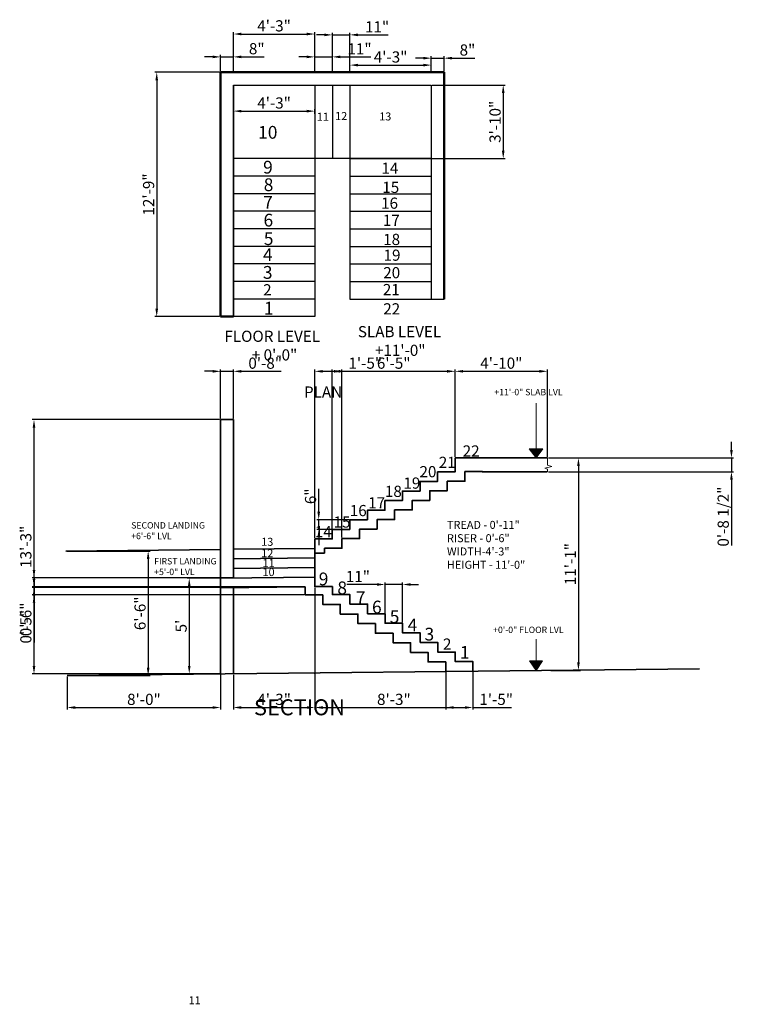
# Model space of a CAD drawing. Units: inches. Extents: x 2958 to 3410, y 1262 to 1879.
import ezdxf

# ---------------------------------------------------------------- set-up
doc = ezdxf.new("R2010")
doc.units = ezdxf.units.IN
for name, color, linetype, lineweight in [('A-ANNO-DIMS', 2, 'Continuous', 18), ('A-ANNO-SYMB', 2, 'Continuous', 18), ('A-ANNO-TEXT', 7, 'Continuous', 18), ('A-FLOR-STRS', 3, 'Continuous', 25), ('A-SECT', 7, 'Continuous', 35), ('A-WALL', 7, 'Continuous', 50)]:
    doc.layers.add(name, color=color, linetype=linetype, lineweight=lineweight)
doc.styles.get("Standard").update_dxf_attribs({"font": 'arial.ttf'})
doc.dimstyles.new('ISO-25', dxfattribs={"dimtxt": 7, "dimasz": 5, "dimexe": 1.25, "dimexo": 0.625, "dimtad": 1, "dimdec": 0, "dimlunit": 3, "dimtxsty": 'Standard', "dimcen": 2.5, "dimadec": 0, "dimazin": 0, "dimtfac": 1, "dimtdec": 0, "dimtmove": 0, "dimatfit": 3, "dimfxl": 1, "dimarcsym": 0})

# ---------------------------------------------------------------- blocks, each defined once
blk = doc.blocks.new('*D1')
at = {"layer": 'A-ANNO-DIMS', "color": 0, "lineweight": -2, "transparency": 16777216}
for p, q in [((3083.14, 1845.78), (3042.51, 1845.78)), ((3043.76, 1840.78), (3043.76, 1697.78)), ((3083.14, 1692.78), (3042.51, 1692.78))]:
    blk.add_line(p, q, dxfattribs=at)
at = {"layer": 'A-ANNO-DIMS', "color": 0, "transparency": 16777216}
for points in [[(3042.92, 1840.78), (3044.59, 1840.78), (3043.76, 1845.78)], [(3042.92, 1697.78), (3044.59, 1697.78), (3043.76, 1692.78)]]:
    blk.add_solid(points, dxfattribs=at)
at = {"layer": 'Defpoints', "color": 0, "transparency": 16777216}
for p in [(3083.76, 1845.78), (3043.76, 1692.78), (3083.76, 1692.78)]:
    blk.add_point(p, dxfattribs=at)
at = {"layer": 'A-ANNO-DIMS', "color": 0, "transparency": 16777216, "insert": (3039.56, 1769.28), "char_height": 7, "attachment_point": 5, "rotation": 90}
blk.add_mtext('12\'-9"', dxfattribs=at)
blk = doc.blocks.new('*D2')
at = {"layer": 'A-ANNO-DIMS', "color": 0, "lineweight": -2, "transparency": 16777216}
for p, q in [((3216.39, 1837.78), (3262.07, 1837.78)), ((3260.82, 1832.78), (3260.82, 1796.78)), ((3216.39, 1791.78), (3262.07, 1791.78))]:
    blk.add_line(p, q, dxfattribs=at)
at = {"layer": 'A-ANNO-DIMS', "color": 0, "transparency": 16777216}
for points in [[(3259.99, 1832.78), (3261.65, 1832.78), (3260.82, 1837.78)], [(3259.99, 1796.78), (3261.65, 1796.78), (3260.82, 1791.78)]]:
    blk.add_solid(points, dxfattribs=at)
at = {"layer": 'Defpoints', "color": 0, "transparency": 16777216}
for p in [(3215.76, 1837.78), (3215.76, 1791.78), (3260.82, 1791.78)]:
    blk.add_point(p, dxfattribs=at)
at = {"layer": 'A-ANNO-DIMS', "color": 0, "transparency": 16777216, "insert": (3256.62, 1814.78), "char_height": 7, "attachment_point": 5, "rotation": 90}
blk.add_mtext('3\'-10"', dxfattribs=at)
blk = doc.blocks.new('*D3')
at = {"layer": 'A-ANNO-DIMS', "color": 0, "lineweight": -2, "transparency": 16777216}
for p, q in [((3091.76, 1819.79), (3091.76, 1822.73)), ((3096.76, 1821.48), (3137.76, 1821.48)), ((3142.76, 1819.79), (3142.76, 1822.73))]:
    blk.add_line(p, q, dxfattribs=at)
at = {"layer": 'A-ANNO-DIMS', "color": 0, "transparency": 16777216}
for points in [[(3096.76, 1822.31), (3096.76, 1820.65), (3091.76, 1821.48)], [(3137.76, 1822.31), (3137.76, 1820.65), (3142.76, 1821.48)]]:
    blk.add_solid(points, dxfattribs=at)
at = {"layer": 'Defpoints', "color": 0, "transparency": 16777216}
for p in [(3091.76, 1819.16), (3142.76, 1821.48), (3142.76, 1819.16)]:
    blk.add_point(p, dxfattribs=at)
at = {"layer": 'A-ANNO-DIMS', "color": 0, "transparency": 16777216, "insert": (3117.26, 1825.68), "char_height": 7, "attachment_point": 5}
blk.add_mtext('4\'-3"', dxfattribs=at)
blk = doc.blocks.new('*D4')
at = {"layer": 'A-ANNO-DIMS', "color": 0, "lineweight": -2, "transparency": 16777216}
for p, q in [((3083.76, 1846.4), (3083.76, 1856.7)), ((3091.76, 1846.4), (3091.76, 1856.7)), ((3078.76, 1855.45), (3073.76, 1855.45)), ((3083.76, 1855.45), (3091.76, 1855.45)), ((3096.76, 1855.45), (3111.07, 1855.45))]:
    blk.add_line(p, q, dxfattribs=at)
at = {"layer": 'A-ANNO-DIMS', "color": 0, "transparency": 16777216}
for points in [[(3078.76, 1856.29), (3078.76, 1854.62), (3083.76, 1855.45)], [(3096.76, 1856.29), (3096.76, 1854.62), (3091.76, 1855.45)]]:
    blk.add_solid(points, dxfattribs=at)
at = {"layer": 'Defpoints', "color": 0, "transparency": 16777216}
for p in [(3091.76, 1855.45), (3083.76, 1845.78), (3091.76, 1845.78)]:
    blk.add_point(p, dxfattribs=at)
at = {"layer": 'A-ANNO-DIMS', "color": 0, "transparency": 16777216, "insert": (3106.41, 1859.65), "char_height": 7, "attachment_point": 5}
blk.add_mtext('8"', dxfattribs=at)
blk = doc.blocks.new('*D5')
at = {"layer": 'A-ANNO-DIMS', "color": 0, "lineweight": -2, "transparency": 16777216}
for p, q in [((3091.76, 1846.4), (3091.76, 1871.01)), ((3096.76, 1869.76), (3137.76, 1869.76)), ((3142.76, 1846.4), (3142.76, 1871.01))]:
    blk.add_line(p, q, dxfattribs=at)
at = {"layer": 'A-ANNO-DIMS', "color": 0, "transparency": 16777216}
for points in [[(3096.76, 1870.6), (3096.76, 1868.93), (3091.76, 1869.76)], [(3137.76, 1870.6), (3137.76, 1868.93), (3142.76, 1869.76)]]:
    blk.add_solid(points, dxfattribs=at)
at = {"layer": 'Defpoints', "color": 0, "transparency": 16777216}
for p in [(3142.76, 1869.76), (3091.76, 1845.78), (3142.76, 1845.78)]:
    blk.add_point(p, dxfattribs=at)
at = {"layer": 'A-ANNO-DIMS', "color": 0, "transparency": 16777216, "insert": (3117.26, 1873.97), "char_height": 7, "attachment_point": 5}
blk.add_mtext('4\'-3"', dxfattribs=at)
blk = doc.blocks.new('*D6')
at = {"layer": 'A-ANNO-DIMS', "color": 0, "lineweight": -2, "transparency": 16777216}
for p, q in [((3142.76, 1846.4), (3142.76, 1856.69)), ((3153.76, 1846.4), (3153.76, 1856.69)), ((3137.76, 1855.44), (3132.76, 1855.44)), ((3142.76, 1855.44), (3153.76, 1855.44)), ((3158.76, 1855.44), (3177.84, 1855.44))]:
    blk.add_line(p, q, dxfattribs=at)
at = {"layer": 'A-ANNO-DIMS', "color": 0, "transparency": 16777216}
for points in [[(3137.76, 1856.27), (3137.76, 1854.61), (3142.76, 1855.44)], [(3158.76, 1856.27), (3158.76, 1854.61), (3153.76, 1855.44)]]:
    blk.add_solid(points, dxfattribs=at)
at = {"layer": 'Defpoints', "color": 0, "transparency": 16777216}
for p in [(3153.76, 1855.44), (3142.76, 1845.78), (3153.76, 1845.78)]:
    blk.add_point(p, dxfattribs=at)
at = {"layer": 'A-ANNO-DIMS', "color": 0, "transparency": 16777216, "insert": (3170.8, 1859.58), "char_height": 7, "attachment_point": 5}
blk.add_mtext('11"', dxfattribs=at)
blk = doc.blocks.new('*D7')
at = {"layer": 'A-ANNO-DIMS', "color": 0, "lineweight": -2, "transparency": 16777216}
for p, q in [((3148.76, 1869.23), (3143.76, 1869.23)), ((3153.76, 1846.4), (3153.76, 1870.48)), ((3153.76, 1869.23), (3164.76, 1869.23)), ((3164.76, 1846.4), (3164.76, 1870.48)), ((3169.76, 1869.23), (3188.84, 1869.23))]:
    blk.add_line(p, q, dxfattribs=at)
at = {"layer": 'A-ANNO-DIMS', "color": 0, "transparency": 16777216}
for points in [[(3148.76, 1870.06), (3148.76, 1868.4), (3153.76, 1869.23)], [(3169.76, 1870.06), (3169.76, 1868.4), (3164.76, 1869.23)]]:
    blk.add_solid(points, dxfattribs=at)
at = {"layer": 'Defpoints', "color": 0, "transparency": 16777216}
for p in [(3164.76, 1869.23), (3153.76, 1845.78), (3164.76, 1845.78)]:
    blk.add_point(p, dxfattribs=at)
at = {"layer": 'A-ANNO-DIMS', "color": 0, "transparency": 16777216, "insert": (3181.8, 1873.37), "char_height": 7, "attachment_point": 5}
blk.add_mtext('11"', dxfattribs=at)
blk = doc.blocks.new('*D8')
at = {"layer": 'A-ANNO-DIMS', "color": 0, "lineweight": -2, "transparency": 16777216}
for p, q in [((3164.76, 1846.4), (3164.76, 1851.54)), ((3169.76, 1850.29), (3210.76, 1850.29)), ((3215.76, 1846.4), (3215.76, 1851.54))]:
    blk.add_line(p, q, dxfattribs=at)
at = {"layer": 'A-ANNO-DIMS', "color": 0, "transparency": 16777216}
for points in [[(3169.76, 1851.12), (3169.76, 1849.46), (3164.76, 1850.29)], [(3210.76, 1851.12), (3210.76, 1849.46), (3215.76, 1850.29)]]:
    blk.add_solid(points, dxfattribs=at)
at = {"layer": 'Defpoints', "color": 0, "transparency": 16777216}
for p in [(3215.76, 1850.29), (3164.76, 1845.78), (3215.76, 1845.78)]:
    blk.add_point(p, dxfattribs=at)
at = {"layer": 'A-ANNO-DIMS', "color": 0, "transparency": 16777216, "insert": (3190.26, 1854.49), "char_height": 7, "attachment_point": 5}
blk.add_mtext('4\'-3"', dxfattribs=at)
blk = doc.blocks.new('*D9')
at = {"layer": 'A-ANNO-DIMS', "color": 0, "lineweight": -2, "transparency": 16777216}
for p, q in [((3215.76, 1846.4), (3215.76, 1855.9)), ((3223.76, 1846.4), (3223.76, 1855.9)), ((3210.76, 1854.65), (3205.76, 1854.65)), ((3215.76, 1854.65), (3223.76, 1854.65)), ((3228.76, 1854.65), (3243.07, 1854.65))]:
    blk.add_line(p, q, dxfattribs=at)
at = {"layer": 'A-ANNO-DIMS', "color": 0, "transparency": 16777216}
for points in [[(3210.76, 1855.48), (3210.76, 1853.81), (3215.76, 1854.65)], [(3228.76, 1855.48), (3228.76, 1853.81), (3223.76, 1854.65)]]:
    blk.add_solid(points, dxfattribs=at)
at = {"layer": 'Defpoints', "color": 0, "transparency": 16777216}
for p in [(3223.76, 1854.65), (3215.76, 1845.78), (3223.76, 1845.78)]:
    blk.add_point(p, dxfattribs=at)
at = {"layer": 'A-ANNO-DIMS', "color": 0, "transparency": 16777216, "insert": (3238.41, 1858.85), "char_height": 7, "attachment_point": 5}
blk.add_mtext('8"', dxfattribs=at)
blk = doc.blocks.new('*D11')
at = {"layer": 'A-ANNO-DIMS', "color": 0, "lineweight": -2, "transparency": 16777216}
for p, q in [((3145.23, 1570.61), (3145.23, 1584.94)), ((3164.07, 1565.61), (3143.98, 1565.61)), ((3145.23, 1559.61), (3145.23, 1565.61)), ((3164.07, 1559.61), (3143.98, 1559.61)), ((3145.23, 1554.61), (3145.23, 1549.61))]:
    blk.add_line(p, q, dxfattribs=at)
at = {"layer": 'A-ANNO-DIMS', "color": 0, "transparency": 16777216}
for points in [[(3144.4, 1570.61), (3146.07, 1570.61), (3145.23, 1565.61)], [(3144.4, 1554.61), (3146.07, 1554.61), (3145.23, 1559.61)]]:
    blk.add_solid(points, dxfattribs=at)
at = {"layer": 'Defpoints', "color": 0, "transparency": 16777216}
for p in [(3145.23, 1565.61), (3164.7, 1565.61), (3164.7, 1559.61)]:
    blk.add_point(p, dxfattribs=at)
at = {"layer": 'A-ANNO-DIMS', "color": 0, "transparency": 16777216, "insert": (3141.03, 1580.28), "char_height": 7, "attachment_point": 5, "rotation": 90}
blk.add_mtext('6"', dxfattribs=at)
blk = doc.blocks.new('*D12')
at = {"layer": 'A-ANNO-DIMS', "color": 0, "lineweight": -2, "transparency": 16777216}
for p, q in [((3181.81, 1525.07), (3162.74, 1525.07)), ((3186.81, 1501.4), (3186.81, 1526.32)), ((3197.81, 1525.07), (3186.81, 1525.07)), ((3197.81, 1501.4), (3197.81, 1526.32)), ((3202.81, 1525.07), (3207.81, 1525.07))]:
    blk.add_line(p, q, dxfattribs=at)
at = {"layer": 'A-ANNO-DIMS', "color": 0, "transparency": 16777216}
for points in [[(3181.81, 1525.9), (3181.81, 1524.24), (3186.81, 1525.07)], [(3202.81, 1525.9), (3202.81, 1524.24), (3197.81, 1525.07)]]:
    blk.add_solid(points, dxfattribs=at)
at = {"layer": 'Defpoints', "color": 0, "transparency": 16777216}
for p in [(3186.81, 1525.07), (3186.81, 1500.78), (3197.81, 1500.78)]:
    blk.add_point(p, dxfattribs=at)
at = {"layer": 'A-ANNO-DIMS', "color": 0, "transparency": 16777216, "insert": (3169.78, 1529.21), "char_height": 7, "attachment_point": 5}
blk.add_mtext('11"', dxfattribs=at)
blk = doc.blocks.new('*D13')
at = {"layer": 'A-ANNO-DIMS', "color": 0, "lineweight": -2, "transparency": 16777216}
for p, q in [((3083.14, 1529.06), (3062.87, 1529.06)), ((3064.12, 1524.06), (3064.12, 1474.06)), ((3083.14, 1469.06), (3062.87, 1469.06))]:
    blk.add_line(p, q, dxfattribs=at)
at = {"layer": 'A-ANNO-DIMS', "color": 0, "transparency": 16777216}
for points in [[(3063.29, 1524.06), (3064.95, 1524.06), (3064.12, 1529.06)], [(3063.29, 1474.06), (3064.95, 1474.06), (3064.12, 1469.06)]]:
    blk.add_solid(points, dxfattribs=at)
at = {"layer": 'Defpoints', "color": 0, "transparency": 16777216}
for p in [(3083.76, 1529.06), (3064.12, 1469.06), (3083.76, 1469.06)]:
    blk.add_point(p, dxfattribs=at)
at = {"layer": 'A-ANNO-DIMS', "color": 0, "transparency": 16777216, "insert": (3059.94, 1499.06), "char_height": 7, "attachment_point": 5, "rotation": 90}
blk.add_mtext("5'", dxfattribs=at)
blk = doc.blocks.new('*D14')
at = {"layer": 'A-ANNO-DIMS', "color": 0, "lineweight": -2, "transparency": 16777216}
for p, q in [((3289.17, 1604.32), (3309.2, 1604.32)), ((3307.95, 1599.32), (3307.95, 1476.3)), ((3290.61, 1471.3), (3309.2, 1471.3))]:
    blk.add_line(p, q, dxfattribs=at)
at = {"layer": 'A-ANNO-DIMS', "color": 0, "transparency": 16777216}
for points in [[(3307.12, 1599.32), (3308.78, 1599.32), (3307.95, 1604.32)], [(3307.12, 1476.3), (3308.78, 1476.3), (3307.95, 1471.3)]]:
    blk.add_solid(points, dxfattribs=at)
at = {"layer": 'Defpoints', "color": 0, "transparency": 16777216}
for p in [(3288.54, 1604.32), (3289.99, 1471.3), (3307.95, 1471.3)]:
    blk.add_point(p, dxfattribs=at)
at = {"layer": 'A-ANNO-DIMS', "color": 0, "transparency": 16777216, "insert": (3303.81, 1537.81), "char_height": 7, "attachment_point": 5, "rotation": 90}
blk.add_mtext('11\'-1"', dxfattribs=at)
blk = doc.blocks.new('*D15')
at = {"layer": 'A-ANNO-DIMS', "color": 0, "lineweight": -2, "transparency": 16777216}
for p, q in [((2987.46, 1546.01), (3039.64, 1546.01)), ((3038.39, 1541.01), (3038.39, 1473.01)), ((2988.31, 1468.01), (3039.64, 1468.01))]:
    blk.add_line(p, q, dxfattribs=at)
at = {"layer": 'A-ANNO-DIMS', "color": 0, "transparency": 16777216}
for points in [[(3037.55, 1541.01), (3039.22, 1541.01), (3038.39, 1546.01)], [(3037.55, 1473.01), (3039.22, 1473.01), (3038.39, 1468.01)]]:
    blk.add_solid(points, dxfattribs=at)
at = {"layer": 'Defpoints', "color": 0, "transparency": 16777216}
for p in [(2986.84, 1546.01), (2987.68, 1468.01), (3038.39, 1468.01)]:
    blk.add_point(p, dxfattribs=at)
at = {"layer": 'A-ANNO-DIMS', "color": 0, "transparency": 16777216, "insert": (3034.19, 1507.01), "char_height": 7, "attachment_point": 5, "rotation": 90}
blk.add_mtext('6\'-6"', dxfattribs=at)
blk = doc.blocks.new('*D18')
at = {"layer": 'A-ANNO-DIMS', "color": 0, "lineweight": -2, "transparency": 16777216}
for p, q in [((3078.76, 1658.55), (3073.76, 1658.55)), ((3083.76, 1628.91), (3083.76, 1659.8)), ((3083.76, 1658.55), (3091.76, 1658.55)), ((3091.76, 1628.91), (3091.76, 1659.8)), ((3096.76, 1658.55), (3121.62, 1658.55))]:
    blk.add_line(p, q, dxfattribs=at)
at = {"layer": 'A-ANNO-DIMS', "color": 0, "transparency": 16777216}
for points in [[(3078.76, 1659.39), (3078.76, 1657.72), (3083.76, 1658.55)], [(3096.76, 1659.39), (3096.76, 1657.72), (3091.76, 1658.55)]]:
    blk.add_solid(points, dxfattribs=at)
at = {"layer": 'Defpoints', "color": 0, "transparency": 16777216}
for p in [(3091.76, 1658.55), (3083.76, 1628.29), (3091.76, 1628.29)]:
    blk.add_point(p, dxfattribs=at)
at = {"layer": 'A-ANNO-DIMS', "color": 0, "transparency": 16777216, "insert": (3111.69, 1662.75), "char_height": 7, "attachment_point": 5}
blk.add_mtext('0\'-8"', dxfattribs=at)
blk = doc.blocks.new('*D19')
at = {"layer": 'A-ANNO-DIMS', "color": 0, "lineweight": -2, "transparency": 16777216}
for p, q in [((3083.14, 1628.29), (2965.61, 1628.29)), ((2966.86, 1474.06), (2966.86, 1623.29)), ((3083.14, 1469.06), (2965.61, 1469.06))]:
    blk.add_line(p, q, dxfattribs=at)
at = {"layer": 'A-ANNO-DIMS', "color": 0, "transparency": 16777216}
for points in [[(2966.03, 1623.29), (2967.69, 1623.29), (2966.86, 1628.29)], [(2966.03, 1474.06), (2967.69, 1474.06), (2966.86, 1469.06)]]:
    blk.add_solid(points, dxfattribs=at)
at = {"layer": 'Defpoints', "color": 0, "transparency": 16777216}
for p in [(2966.86, 1628.29), (3083.76, 1628.29), (3083.76, 1469.06)]:
    blk.add_point(p, dxfattribs=at)
at = {"layer": 'A-ANNO-DIMS', "color": 0, "transparency": 16777216, "insert": (2962.66, 1548.67), "char_height": 7, "attachment_point": 5, "rotation": 90}
blk.add_mtext('13\'-3"', dxfattribs=at)
blk = doc.blocks.new('*D20')
at = {"layer": 'A-ANNO-DIMS', "color": 0, "lineweight": -2, "transparency": 16777216}
for p, q in [((2987.68, 1467.39), (2987.68, 1446.79)), ((3083.76, 1468.43), (3083.76, 1446.79)), ((2992.68, 1448.04), (3078.76, 1448.04))]:
    blk.add_line(p, q, dxfattribs=at)
at = {"layer": 'A-ANNO-DIMS', "color": 0, "transparency": 16777216}
for points in [[(2992.68, 1448.87), (2992.68, 1447.21), (2987.68, 1448.04)], [(3078.76, 1448.87), (3078.76, 1447.21), (3083.76, 1448.04)]]:
    blk.add_solid(points, dxfattribs=at)
at = {"layer": 'Defpoints', "color": 0, "transparency": 16777216}
for p in [(2987.68, 1468.01), (3083.76, 1469.06), (3083.76, 1448.04)]:
    blk.add_point(p, dxfattribs=at)
at = {"layer": 'A-ANNO-DIMS', "color": 0, "transparency": 16777216, "insert": (3035.72, 1452.24), "char_height": 7, "attachment_point": 5}
blk.add_mtext('8\'-0"', dxfattribs=at)
blk = doc.blocks.new('*D21')
at = {"layer": 'A-ANNO-DIMS', "color": 0, "lineweight": -2, "transparency": 16777216}
for p, q in [((3142.83, 1523.08), (3142.83, 1446.79)), ((3091.76, 1468.43), (3091.76, 1446.79)), ((3096.76, 1448.04), (3137.83, 1448.04))]:
    blk.add_line(p, q, dxfattribs=at)
at = {"layer": 'A-ANNO-DIMS', "color": 0, "transparency": 16777216}
for points in [[(3096.76, 1448.87), (3096.76, 1447.21), (3091.76, 1448.04)], [(3137.83, 1448.87), (3137.83, 1447.21), (3142.83, 1448.04)]]:
    blk.add_solid(points, dxfattribs=at)
at = {"layer": 'Defpoints', "color": 0, "transparency": 16777216}
for p in [(3142.83, 1523.71), (3091.76, 1469.06), (3142.83, 1448.04)]:
    blk.add_point(p, dxfattribs=at)
at = {"layer": 'A-ANNO-DIMS', "color": 0, "transparency": 16777216, "insert": (3117.29, 1452.24), "char_height": 7, "attachment_point": 5}
blk.add_mtext('4\'-3"', dxfattribs=at)
blk = doc.blocks.new('*D22')
at = {"layer": 'A-ANNO-DIMS', "color": 0, "lineweight": -2, "transparency": 16777216}
for p, q in [((3142.83, 1523.08), (3142.83, 1446.79)), ((3241.81, 1470.15), (3241.81, 1446.79)), ((3147.83, 1448.04), (3236.81, 1448.04))]:
    blk.add_line(p, q, dxfattribs=at)
at = {"layer": 'A-ANNO-DIMS', "color": 0, "transparency": 16777216}
for points in [[(3147.83, 1448.87), (3147.83, 1447.21), (3142.83, 1448.04)], [(3236.81, 1448.87), (3236.81, 1447.21), (3241.81, 1448.04)]]:
    blk.add_solid(points, dxfattribs=at)
at = {"layer": 'Defpoints', "color": 0, "transparency": 16777216}
for p in [(3142.83, 1523.71), (3241.81, 1470.78), (3241.81, 1448.04)]:
    blk.add_point(p, dxfattribs=at)
at = {"layer": 'A-ANNO-DIMS', "color": 0, "transparency": 16777216, "insert": (3192.32, 1452.24), "char_height": 7, "attachment_point": 5}
blk.add_mtext('8\'-3"', dxfattribs=at)
blk = doc.blocks.new('*D23')
at = {"layer": 'A-ANNO-DIMS', "color": 0, "lineweight": -2, "transparency": 16777216}
for p, q in [((3224.77, 1469.97), (3224.77, 1446.79)), ((3241.81, 1470.15), (3241.81, 1446.79)), ((3229.77, 1448.04), (3236.81, 1448.04)), ((3241.81, 1448.04), (3266.01, 1448.04))]:
    blk.add_line(p, q, dxfattribs=at)
at = {"layer": 'A-ANNO-DIMS', "color": 0, "transparency": 16777216}
for points in [[(3229.77, 1448.87), (3229.77, 1447.21), (3224.77, 1448.04)], [(3236.81, 1448.87), (3236.81, 1447.21), (3241.81, 1448.04)]]:
    blk.add_solid(points, dxfattribs=at)
at = {"layer": 'Defpoints', "color": 0, "transparency": 16777216}
for p in [(3224.77, 1470.59), (3241.81, 1470.78), (3241.81, 1448.04)]:
    blk.add_point(p, dxfattribs=at)
at = {"layer": 'A-ANNO-DIMS', "color": 0, "transparency": 16777216, "insert": (3256.41, 1452.24), "char_height": 7, "attachment_point": 5}
blk.add_mtext('1\'-5"', dxfattribs=at)
blk = doc.blocks.new('*D24')
at = {"layer": 'A-ANNO-DIMS', "color": 0, "lineweight": -2, "transparency": 16777216}
for p, q in [((2966.86, 1534.15), (2966.86, 1539.15)), ((3091.14, 1529.15), (2965.61, 1529.15)), ((2966.86, 1529.15), (2966.86, 1523.15)), ((3091.14, 1523.15), (2965.61, 1523.15)), ((2966.86, 1518.15), (2966.86, 1493.29))]:
    blk.add_line(p, q, dxfattribs=at)
at = {"layer": 'A-ANNO-DIMS', "color": 0, "transparency": 16777216}
for points in [[(2966.03, 1534.15), (2967.69, 1534.15), (2966.86, 1529.15)], [(2966.03, 1518.15), (2967.69, 1518.15), (2966.86, 1523.15)]]:
    blk.add_solid(points, dxfattribs=at)
at = {"layer": 'Defpoints', "color": 0, "transparency": 16777216}
for p in [(3091.76, 1529.15), (2966.86, 1523.15), (3091.76, 1523.15)]:
    blk.add_point(p, dxfattribs=at)
at = {"layer": 'A-ANNO-DIMS', "color": 0, "transparency": 16777216, "insert": (2962.66, 1503.22), "char_height": 7, "attachment_point": 5, "rotation": 90}
blk.add_mtext('0\'-6"', dxfattribs=at)
blk = doc.blocks.new('*D25')
at = {"layer": 'A-ANNO-DIMS', "color": 0, "lineweight": -2, "transparency": 16777216}
for p, q in [((2966.86, 1528.58), (2966.86, 1533.58)), ((3136.15, 1523.58), (2965.61, 1523.58)), ((2966.86, 1523.58), (2966.86, 1518.59)), ((3136.14, 1518.59), (2965.61, 1518.59)), ((2966.86, 1513.59), (2966.86, 1488.74))]:
    blk.add_line(p, q, dxfattribs=at)
at = {"layer": 'A-ANNO-DIMS', "color": 0, "transparency": 16777216}
for points in [[(2966.03, 1528.58), (2967.69, 1528.58), (2966.86, 1523.58)], [(2966.03, 1513.59), (2967.69, 1513.59), (2966.86, 1518.59)]]:
    blk.add_solid(points, dxfattribs=at)
at = {"layer": 'Defpoints', "color": 0, "transparency": 16777216}
for p in [(3136.78, 1523.58), (2966.86, 1518.59), (3136.77, 1518.59)]:
    blk.add_point(p, dxfattribs=at)
at = {"layer": 'A-ANNO-DIMS', "color": 0, "transparency": 16777216, "insert": (2962.66, 1498.66), "char_height": 7, "attachment_point": 5, "rotation": 90}
blk.add_mtext('0\'-5"', dxfattribs=at)
blk = doc.blocks.new('*D26')
at = {"layer": 'A-ANNO-DIMS', "color": 0, "lineweight": -2, "transparency": 16777216}
for p, q in [((3153.7, 1560.23), (3153.7, 1659.8)), ((3158.7, 1658.55), (3225.7, 1658.55)), ((3230.7, 1604.95), (3230.7, 1659.8))]:
    blk.add_line(p, q, dxfattribs=at)
at = {"layer": 'A-ANNO-DIMS', "color": 0, "transparency": 16777216}
for points in [[(3158.7, 1659.39), (3158.7, 1657.72), (3153.7, 1658.55)], [(3225.7, 1659.39), (3225.7, 1657.72), (3230.7, 1658.55)]]:
    blk.add_solid(points, dxfattribs=at)
at = {"layer": 'Defpoints', "color": 0, "transparency": 16777216}
for p in [(3230.7, 1658.55), (3230.7, 1604.32), (3153.7, 1559.61)]:
    blk.add_point(p, dxfattribs=at)
at = {"layer": 'A-ANNO-DIMS', "color": 0, "transparency": 16777216, "insert": (3192.2, 1662.75), "char_height": 7, "attachment_point": 5}
blk.add_mtext('6\'-5"', dxfattribs=at)
blk = doc.blocks.new('*D27')
at = {"layer": 'A-ANNO-DIMS', "color": 0, "lineweight": -2, "transparency": 16777216}
for p, q in [((3230.7, 1604.95), (3230.7, 1659.8)), ((3235.7, 1658.55), (3283.54, 1658.55)), ((3288.54, 1604.95), (3288.54, 1659.8))]:
    blk.add_line(p, q, dxfattribs=at)
at = {"layer": 'A-ANNO-DIMS', "color": 0, "transparency": 16777216}
for points in [[(3235.7, 1659.39), (3235.7, 1657.72), (3230.7, 1658.55)], [(3283.54, 1659.39), (3283.54, 1657.72), (3288.54, 1658.55)]]:
    blk.add_solid(points, dxfattribs=at)
at = {"layer": 'Defpoints', "color": 0, "transparency": 16777216}
for p in [(3288.54, 1658.55), (3230.7, 1604.32), (3288.54, 1604.32)]:
    blk.add_point(p, dxfattribs=at)
at = {"layer": 'A-ANNO-DIMS', "color": 0, "transparency": 16777216, "insert": (3259.62, 1662.75), "char_height": 7, "attachment_point": 5}
blk.add_mtext('4\'-10"', dxfattribs=at)
blk = doc.blocks.new('*D28')
at = {"layer": 'A-ANNO-DIMS', "color": 0, "lineweight": -2, "transparency": 16777216}
for p, q in [((3142.76, 1554.23), (3142.76, 1659.8)), ((3147.76, 1658.55), (3154.79, 1658.55)), ((3159.79, 1554.4), (3159.79, 1659.8)), ((3159.79, 1658.55), (3183.99, 1658.55))]:
    blk.add_line(p, q, dxfattribs=at)
at = {"layer": 'A-ANNO-DIMS', "color": 0, "transparency": 16777216}
for points in [[(3147.76, 1659.39), (3147.76, 1657.72), (3142.76, 1658.55)], [(3154.79, 1659.39), (3154.79, 1657.72), (3159.79, 1658.55)]]:
    blk.add_solid(points, dxfattribs=at)
at = {"layer": 'Defpoints', "color": 0, "transparency": 16777216}
for p in [(3159.79, 1658.55), (3159.79, 1553.77), (3142.76, 1553.61)]:
    blk.add_point(p, dxfattribs=at)
at = {"layer": 'A-ANNO-DIMS', "color": 0, "transparency": 16777216, "insert": (3174.39, 1662.75), "char_height": 7, "attachment_point": 5}
blk.add_mtext('1\'-5"', dxfattribs=at)
blk = doc.blocks.new('*D29')
at = {"layer": 'A-ANNO-DIMS', "color": 0, "lineweight": -2, "transparency": 16777216}
for p, q in [((3403.79, 1609.32), (3403.79, 1614.32)), ((3289.17, 1604.32), (3405.04, 1604.32)), ((3403.79, 1604.32), (3403.79, 1595.67)), ((3289.26, 1595.67), (3405.04, 1595.67)), ((3403.79, 1590.67), (3403.79, 1549.5))]:
    blk.add_line(p, q, dxfattribs=at)
at = {"layer": 'A-ANNO-DIMS', "color": 0, "transparency": 16777216}
for points in [[(3402.95, 1609.32), (3404.62, 1609.32), (3403.79, 1604.32)], [(3402.95, 1590.67), (3404.62, 1590.67), (3403.79, 1595.67)]]:
    blk.add_solid(points, dxfattribs=at)
at = {"layer": 'Defpoints', "color": 0, "transparency": 16777216}
for p in [(3288.54, 1604.32), (3288.63, 1595.67), (3403.79, 1595.67)]:
    blk.add_point(p, dxfattribs=at)
at = {"layer": 'A-ANNO-DIMS', "color": 0, "transparency": 16777216, "insert": (3399.54, 1567.59), "char_height": 7, "attachment_point": 5, "rotation": 90}
blk.add_mtext('0\'-8 1/2"', dxfattribs=at)

msp = doc.modelspace()

# ---------------------------------------------------------------- hatches: boundary and pattern name
at = {"layer": 'A-ANNO-SYMB'}
h = msp.add_hatch(color=256, dxfattribs=at)
h.dxf.hatch_style = 1
h.paths.add_polyline_path([(3281.39, 1604.32), (3281.39, 1610.09), (3277.15, 1610.09)])
h = msp.add_hatch(color=256, dxfattribs=at)
h.dxf.hatch_style = 1
h.paths.add_polyline_path([(3281.39, 1610.09), (3281.39, 1604.32), (3285.63, 1610.09)])
h = msp.add_hatch(color=256, dxfattribs=at)
h.dxf.hatch_style = 1
h.paths.add_polyline_path([(3281.39, 1477.29), (3277.33, 1477.29), (3281.39, 1471.23)])
h = msp.add_hatch(color=256, dxfattribs=at)
h.dxf.hatch_style = 1
h.paths.add_polyline_path([(3284.97, 1476.51), (3285.49, 1477.29), (3281.39, 1477.29), (3281.39, 1471.23), (3281.4, 1471.22)])

# ---------------------------------------------------------------- linework, layer by layer
for p, q in [((3281.39, 1604.32), (3281.39, 1638.58)), ((3281.39, 1604.32), (3277.15, 1610.09)), ((3277.15, 1610.09), (3285.63, 1610.09)), ((3281.39, 1604.32), (3285.63, 1610.09)), ((3281.39, 1604.32), (3281.39, 1604.32)), ((3288.54, 1604.32), (3288.54, 1599.77)), ((3291.35, 1598.97), (3286.82, 1598.01)), ((3286.82, 1598.01), (3288.63, 1597.26)), ((3288.54, 1599.77), (3291.35, 1598.97)), ((3288.63, 1597.26), (3288.63, 1595.67)), ((3281.39, 1471.21), (3281.39, 1490.93)), ((3281.41, 1471.19), (3277.33, 1477.29)), ((3277.33, 1477.29), (3285.49, 1477.29)), ((3281.39, 1471.21), (3285.49, 1477.28)), ((3281.41, 1471.19), (3285.49, 1477.29))]:
    msp.add_line(p, q, dxfattribs=at)
at = {"layer": 'A-FLOR-STRS'}
for p, q in [((3091.76, 1692.78), (3091.76, 1837.78)), ((3091.76, 1837.78), (3142.76, 1837.78)), ((3091.76, 1837.78), (3091.76, 1692.78)), ((3142.76, 1837.78), (3142.76, 1692.78)), ((3142.76, 1837.78), (3153.76, 1837.78)), ((3142.76, 1837.78), (3142.76, 1692.78)), ((3153.76, 1837.78), (3164.76, 1837.78)), ((3153.76, 1837.78), (3153.76, 1791.78)), ((3164.76, 1837.78), (3215.76, 1837.78)), ((3164.76, 1837.78), (3164.76, 1703.78)), ((3215.76, 1837.78), (3215.76, 1703.78)), ((3215.76, 1791.78), (3091.76, 1791.78)), ((3164.76, 1791.78), (3215.76, 1791.78)), ((3142.76, 1780.78), (3091.76, 1780.78)), ((3164.76, 1780.78), (3215.76, 1780.78)), ((3142.76, 1769.78), (3091.76, 1769.78)), ((3164.76, 1769.78), (3215.76, 1769.78)), ((3142.76, 1758.78), (3091.76, 1758.78)), ((3164.76, 1758.78), (3215.76, 1758.78)), ((3142.76, 1747.78), (3091.76, 1747.78)), ((3164.76, 1747.78), (3215.76, 1747.78)), ((3142.76, 1736.78), (3091.76, 1736.78)), ((3164.76, 1736.78), (3215.76, 1736.78)), ((3142.76, 1725.78), (3091.76, 1725.78)), ((3164.76, 1725.78), (3215.76, 1725.78)), ((3142.76, 1714.78), (3091.76, 1714.78)), ((3164.76, 1714.78), (3215.76, 1714.78)), ((3142.76, 1703.78), (3091.76, 1703.78)), ((3164.76, 1703.78), (3223.76, 1703.78)), ((3142.76, 1692.78), (3091.76, 1692.78))]:
    msp.add_line(p, q, dxfattribs=at)
at = {"layer": 'A-SECT'}
for p, q in [((3083.76, 1628.29), (3083.76, 1469.06)), ((3083.76, 1628.29), (3091.76, 1628.29)), ((3091.76, 1628.29), (3091.76, 1529.15)), ((3230.7, 1604.32), (3288.54, 1604.32)), ((3230.7, 1601.61), (3230.7, 1604.32)), ((3247.7, 1595.67), (3288.41, 1595.67)), ((3083.4, 1562.06), (3083.76, 1562.07)), ((3083.52, 1551.06), (3083.76, 1551.06)), ((3091.76, 1547.15), (3142.76, 1547.71)), ((3142.7, 1551.71), (3142.76, 1551.71)), ((3142.76, 1553.61), (3142.76, 1529.71)), ((3148.79, 1544.77), (3148.79, 1547.77)), ((2986.84, 1546.01), (3083.76, 1547.06)), ((3091.76, 1541.15), (3142.63, 1541.7)), ((3142.76, 1544.71), (3148.79, 1544.77)), ((3142.76, 1544.71), (3142.79, 1544.71)), ((3083.63, 1541.06), (3083.76, 1541.06)), ((3083.64, 1540.06), (3083.76, 1540.06)), ((3091.76, 1535.15), (3142.7, 1535.7)), ((3083.7, 1535.06), (3083.76, 1535.06)), ((3083.76, 1529.06), (3142.76, 1529.71)), ((3142.76, 1529.71), (3142.83, 1523.71)), ((3083.76, 1523.06), (3136.77, 1523.64)), ((3091.76, 1523.15), (3091.76, 1469.06)), ((3136.78, 1523.58), (3125.78, 1523.58)), ((3142.83, 1523.71), (3153.81, 1523.83)), ((3153.83, 1523.77), (3142.83, 1523.77)), ((2987.68, 1468.01), (3383.81, 1472.32)), ((3142.76, 1469.7), (3142.76, 1469.06))]:
    msp.add_line(p, q, dxfattribs=at)
for points in [[(3142.7, 1547.61), (3142.7, 1553.61), (3153.7, 1553.61), (3153.7, 1559.61), (3164.7, 1559.61), (3164.7, 1565.61), (3175.7, 1565.61), (3175.7, 1571.61), (3186.7, 1571.61), (3186.7, 1577.61), (3197.7, 1577.61), (3197.7, 1583.61), (3208.7, 1583.61), (3208.7, 1589.61), (3219.7, 1589.61), (3219.7, 1595.61), (3230.7, 1595.61), (3230.7, 1601.61)], [(3148.79, 1547.77), (3159.79, 1547.77), (3159.79, 1553.77), (3170.79, 1553.77), (3170.79, 1559.77), (3181.79, 1559.77), (3181.79, 1565.77), (3192.79, 1565.77), (3192.79, 1571.77), (3203.79, 1571.77), (3203.79, 1577.77), (3214.79, 1577.77), (3214.79, 1583.77), (3225.79, 1583.77), (3225.79, 1589.77), (3236.79, 1589.77), (3236.79, 1595.77), (3247.79, 1595.77)], [(3224.77, 1470.59), (3224.77, 1476.59), (3213.77, 1476.59), (3213.77, 1482.59), (3202.77, 1482.59), (3202.77, 1488.59), (3191.77, 1488.59), (3191.77, 1494.59), (3180.77, 1494.59), (3180.77, 1500.59), (3169.77, 1500.59), (3169.77, 1506.59), (3158.77, 1506.59), (3158.77, 1512.59), (3147.77, 1512.59), (3147.77, 1518.59), (3136.77, 1518.59), (3136.77, 1523.64)], [(3241.81, 1470.78), (3241.81, 1476.78), (3230.81, 1476.78), (3230.81, 1482.78), (3219.81, 1482.78), (3219.81, 1488.78), (3208.81, 1488.78), (3208.81, 1494.78), (3197.81, 1494.78), (3197.81, 1500.78), (3186.81, 1500.78), (3186.81, 1506.78), (3175.81, 1506.78), (3175.81, 1512.78), (3164.81, 1512.78), (3164.81, 1518.78), (3153.81, 1518.78), (3153.81, 1523.83)]]:
    msp.add_lwpolyline(points, dxfattribs=at)
at = {"layer": 'A-WALL'}
for p, q in [((3083.76, 1845.78), (3083.76, 1692.78)), ((3223.76, 1845.78), (3083.76, 1845.78)), ((3223.76, 1703.78), (3223.76, 1845.78)), ((3083.76, 1692.78), (3091.76, 1692.78))]:
    msp.add_line(p, q, dxfattribs=at)

# ---------------------------------------------------------------- texts
at = {"layer": 'A-ANNO-TEXT', "attachment_point": 1}
for s, width, heights, insert, char_height in [('11', 41.8662, [0], (3144.03, 1820.48), 5), ('12', 41.8662, [0], (3155.51, 1820.92), 5), ('13', 41.8662, [0], (3183.12, 1820.65), 5), ('10', 41.8662, [0], (3107.25, 1812.21), 8), ('9', 41.8662, [0], (3110.4, 1790.37), 8), ('14', 41.8662, [0], (3184.52, 1789.25), 7), ('8', 41.8662, [0], (3110.76, 1779.39), 8), ('15', 41.8662, [0], (3185.05, 1777.25), 7), ('7', 41.8662, [0], (3110.46, 1768.36), 8), ('16', 41.8662, [0], (3184.3, 1767.36), 7), ('6', 41.8662, [0], (3110.64, 1757.21), 8), ('17', 41.8662, [0], (3185.45, 1756.64), 7), ('5', 41.8662, [0], (3110.83, 1745.63), 8), ('18', 41.8662, [0], (3185.61, 1744.64), 7), ('4', 41.8662, [0], (3110.33, 1735.55), 8), ('19', 41.8662, [0], (3185.85, 1734.77), 7), ('3', 41.8662, [0], (3110.25, 1724.49), 8), ('20', 41.8662, [0], (3185.64, 1723.82), 7), ('2', 41.8662, [0], (3110.41, 1713.12), 7), ('21', 41.8662, [0], (3185.4, 1713.23), 7), ('1', 41.8662, [0], (3110.91, 1702.07), 8), ('22', 41.8662, [0], (3185.66, 1701.18), 7), ('{\\fArial|b1|i0|c0|p34;FLOOR LEVEL\\P        + 0\'-0"}', 78.9075, [28.19], (3086.15, 1684), 7), ('{\\fArial|b1|i0|c0|p34;SLAB LEVEL\\P     +11\'-0"}', 69.0443, [27.81], (3169.76, 1686.88), 7), ('{\\fArial|b1|i0|c0|p34;PLAN}', 41.8662, [0], (3136, 1649.09), 7), ('{\\fArial|b1|i0|c0|p34;+11\'-0" SLAB LVL}', 66.0826, [0], (3255.26, 1647.55), 4), ('22', 41.8662, [0], (3235.42, 1612.18), 7), ('21', 41.8662, [0], (3220.46, 1605.04), 7), ('20', 41.8662, [0], (3208.35, 1599.2), 7), ('19', 41.8662, [0], (3198.27, 1592.07), 7), ('18', 41.8662, [0], (3186.7, 1586.89), 7), ('17', 41.8662, [0], (3176.25, 1579.74), 7), ('16', 41.8662, [0], (3164.7, 1574.86), 7), ('15', 41.8662, [0], (3154.55, 1567.71), 7), ('14', 41.8662, [0], (3142.81, 1561.64), 7), ('{\\fArial|b1|i0|c0|p34;TREAD - 0\'-11"\\PRISER - 0\'-6"\\PWIDTH-4\'-3"\\PHEIGHT - 11\'-0"}', 66.4887, [42.14], (3225.59, 1564.91), 5), ('13', 41.8662, [0], (3109.2, 1554.3), 5), ('{\\fArial|b1|i0|c0|p34;FIRST LANDING +5\'-0" LVL}', 54.0253, [25.57], (3042.14, 1541.63), 4), ('12', 41.8662, [0], (3109.2, 1547.14), 5), ('11', 41.8662, [0], (3110.02, 1540.98), 5), ('10', 41.8662, [0], (3110.02, 1535.35), 5), ('9', 41.8662, [0], (3145.25, 1532.55), 8), ('8', 41.8662, [0], (3156.9, 1526.95), 8), ('7', 41.8662, [0], (3168.47, 1520.78), 8), ('6', 41.8662, [0], (3178.61, 1514.95), 8), ('5', 41.8662, [0], (3189.72, 1508.92), 8), ('4', 41.8662, [0], (3200.97, 1503.74), 8), ('{\\fArial|b1|i0|c0|p34;+0\'-0" FLOOR LVL}', 66.0826, [0], (3254.49, 1498.68), 4), ('3', 41.8662, [0], (3211.51, 1497.98), 8), ('2', 41.8662, [0], (3223.06, 1491.26), 7), ('1', 41.8662, [0], (3233.66, 1486.56), 8), ('{\\fArial|b1|i0|c0|p34;SECTION }', 137.5792, [0], (3104.68, 1453.18), 10), ('11', 41.8662, [0], (3063.71, 1267.2), 5)]:
    msp.add_mtext_dynamic_manual_height_columns(s, width=width, gutter_width=12.5, heights=heights, dxfattribs=dict(at, insert=insert, char_height=char_height))
at = {"layer": 'A-ANNO-TEXT', "insert": (3027.74, 1564.11), "char_height": 4, "width": 72.7809, "attachment_point": 1}
msp.add_mtext('{\\fArial|b1|i0|c0|p34;SECOND LANDING\\P+6\'-6" LVL}', dxfattribs=at)

# ---------------------------------------------------------------- dimensions: what is measured, and where the dimension line sits
at = {"layer": 'A-ANNO-DIMS'}
for base, p1, p2, override, picture, middle in [((3142.76, 1869.76), (3091.76, 1845.78), (3142.76, 1845.78), {"dimclrd": 0, "dimclre": 0, "dimclrt": 0}, '*D5', (3117.26, 1873.97)), ((3164.76, 1869.23), (3153.76, 1845.78), (3164.76, 1845.78), {"dimclrd": 0, "dimclre": 0, "dimclrt": 0}, '*D7', (3181.8, 1873.37)), ((3091.76, 1855.45), (3083.76, 1845.78), (3091.76, 1845.78), {"dimclrd": 0, "dimclre": 0, "dimclrt": 0}, '*D4', (3106.41, 1859.65)), ((3153.76, 1855.44), (3142.76, 1845.78), (3153.76, 1845.78), {"dimclrd": 0, "dimclre": 0, "dimclrt": 0}, '*D6', (3170.8, 1859.58)), ((3223.76, 1854.65), (3215.76, 1845.78), (3223.76, 1845.78), {"dimclrd": 0, "dimclre": 0, "dimclrt": 0}, '*D9', (3238.41, 1858.85)), ((3215.76, 1850.29), (3164.76, 1845.78), (3215.76, 1845.78), {"dimclrd": 0, "dimclre": 0, "dimclrt": 0}, '*D8', (3190.26, 1854.49)), ((3142.76, 1821.48), (3091.76, 1819.16), (3142.76, 1819.16), {"dimclrd": 0, "dimclre": 0, "dimclrt": 0}, '*D3', (3117.26, 1825.68)), ((3091.76, 1658.55), (3083.76, 1628.29), (3091.76, 1628.29), {"dimdec": 1, "dimlfac": 1, "dimrnd": 0, "dimzin": 1, "dimdsep": 46, "dimlunit": 4, "dimfrac": 2}, '*D18', (3111.69, 1662.75)), ((3159.79, 1658.55), (3142.76, 1553.61), (3159.79, 1553.77), {"dimdec": 1, "dimlfac": 1, "dimrnd": 0, "dimzin": 1, "dimdsep": 46, "dimlunit": 4, "dimfrac": 2}, '*D28', (3174.39, 1662.75)), ((3230.7, 1658.55), (3153.7, 1559.61), (3230.7, 1604.32), {"dimdec": 1, "dimlfac": 1, "dimrnd": 0, "dimzin": 1, "dimdsep": 46, "dimlunit": 4, "dimfrac": 2}, '*D26', (3192.2, 1662.75)), ((3288.54, 1658.55), (3230.7, 1604.32), (3288.54, 1604.32), {"dimdec": 1, "dimlfac": 1, "dimrnd": 0, "dimzin": 1, "dimdsep": 46, "dimlunit": 4, "dimfrac": 2}, '*D27', (3259.62, 1662.75)), ((3186.81, 1525.07), (3197.81, 1500.78), (3186.81, 1500.78), {"dimclrd": 0, "dimclre": 0, "dimclrt": 0}, '*D12', (3169.78, 1529.21)), ((3142.83, 1448.04), (3091.76, 1469.06), (3142.83, 1523.71), {"dimdec": 1, "dimlfac": 1, "dimrnd": 0, "dimzin": 1, "dimdsep": 46, "dimlunit": 4, "dimfrac": 2}, '*D21', (3117.29, 1452.24)), ((3241.81, 1448.04), (3142.83, 1523.71), (3241.81, 1470.78), {"dimdec": 1, "dimlfac": 1, "dimrnd": 0, "dimzin": 1, "dimdsep": 46, "dimlunit": 4, "dimfrac": 2}, '*D22', (3192.32, 1452.24)), ((3083.76, 1448.04), (2987.68, 1468.01), (3083.76, 1469.06), {"dimdec": 1, "dimlfac": 1, "dimrnd": 0, "dimzin": 1, "dimdsep": 46, "dimlunit": 4, "dimfrac": 2}, '*D20', (3035.72, 1452.24)), ((3241.81, 1448.04), (3224.77, 1470.59), (3241.81, 1470.78), {"dimdec": 1, "dimlfac": 1, "dimrnd": 0, "dimzin": 1, "dimdsep": 46, "dimlunit": 4, "dimfrac": 2}, '*D23', (3256.41, 1452.24))]:
    dim = msp.add_linear_dim(base=base, p1=p1, p2=p2, dimstyle='ISO-25', override=override, dxfattribs=at)
    dim.commit()
    dim.dimension.update_dxf_attribs({"geometry": picture, "text_midpoint": middle})
for base, p1, p2, override, picture, middle in [((3043.76, 1692.78), (3083.76, 1845.78), (3083.76, 1692.78), {"dimclrd": 0, "dimclre": 0, "dimclrt": 0}, '*D1', (3039.56, 1769.28)), ((3260.82, 1791.78), (3215.76, 1837.78), (3215.76, 1791.78), {"dimclrd": 0, "dimclre": 0, "dimclrt": 0}, '*D2', (3256.62, 1814.78)), ((2966.86, 1628.29), (3083.76, 1469.06), (3083.76, 1628.29), {"dimdec": 1, "dimlfac": 1, "dimrnd": 0, "dimzin": 1, "dimdsep": 46, "dimlunit": 4, "dimfrac": 2}, '*D19', (2962.66, 1548.67)), ((3403.7864, 1595.6735), (3288.5426, 1604.3237), (3288.6318, 1595.6735), {"dimdec": 1, "dimlfac": 1, "dimrnd": 0, "dimzin": 1, "dimdsep": 46, "dimlunit": 4, "dimfrac": 2}, '*D29', (3399.542, 1567.5891)), ((3307.95, 1471.3), (3288.54, 1604.32), (3289.99, 1471.3), {"dimclrd": 0, "dimclre": 0, "dimclrt": 0}, '*D14', (3303.81, 1537.81)), ((3145.23, 1565.61), (3164.7, 1559.61), (3164.7, 1565.61), {"dimclrd": 0, "dimclre": 0, "dimclrt": 0}, '*D11', (3141.03, 1580.28)), ((3038.39, 1468.01), (2986.84, 1546.01), (2987.68, 1468.01), {"dimclrd": 0, "dimclre": 0, "dimclrt": 0}, '*D15', (3034.19, 1507.01)), ((2966.86, 1523.15), (3091.76, 1529.15), (3091.76, 1523.15), {"dimdec": 1, "dimlfac": 1, "dimrnd": 0, "dimzin": 1, "dimdsep": 46, "dimlunit": 4, "dimfrac": 2}, '*D24', (2962.66, 1503.22)), ((2966.86, 1518.59), (3136.78, 1523.58), (3136.77, 1518.59), {"dimdec": 1, "dimlfac": 1, "dimrnd": 0, "dimzin": 1, "dimdsep": 46, "dimlunit": 4, "dimfrac": 2}, '*D25', (2962.66, 1498.66)), ((3064.12, 1469.06), (3083.76, 1529.06), (3083.76, 1469.06), {"dimclrd": 0, "dimclre": 0, "dimclrt": 0}, '*D13', (3059.94, 1499.06))]:
    dim = msp.add_linear_dim(base=base, p1=p1, p2=p2, angle=90, dimstyle='ISO-25', override=override, dxfattribs=at)
    dim.commit()
    dim.dimension.update_dxf_attribs({"geometry": picture, "text_midpoint": middle})

doc.saveas('drawing.dxf')
